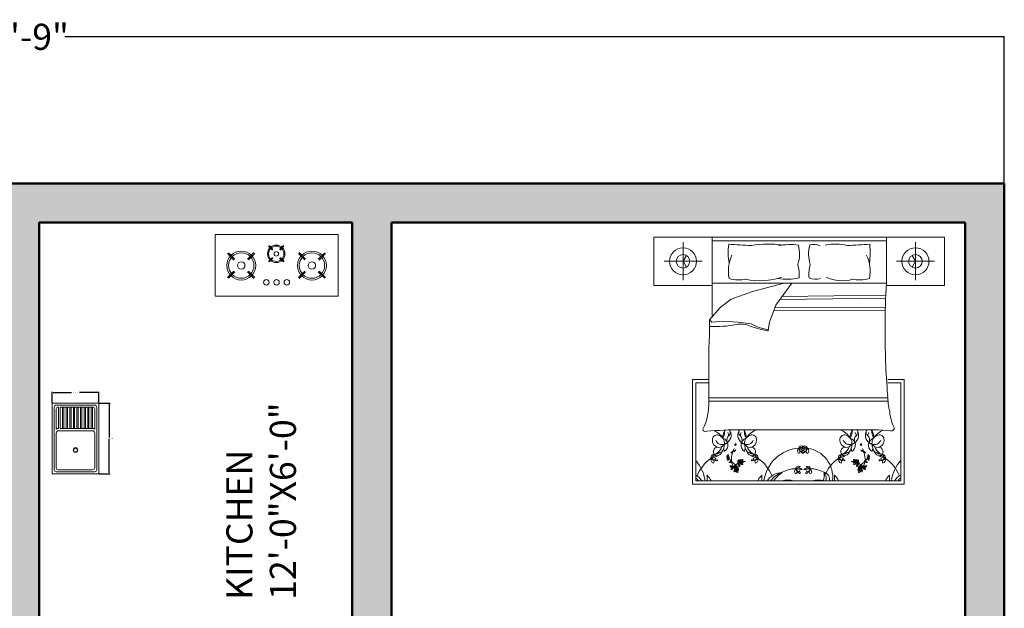
# Model space of a CAD drawing. Units: inches. Extents: x -17 to 536, y -817 to 53.
# Tile 9 of 9: x 268 to 494, y -86 to 49. Entities that reach past the tile are written whole.
import ezdxf

# ---------------------------------------------------------------- set-up
doc = ezdxf.new("R2010")
doc.units = ezdxf.units.IN
doc.header["$MEASUREMENT"] = 0
for name, color, linetype, lineweight in [('A-ANNO-DIMS', 2, 'Continuous', 18), ('A-AREA-IDEN', 7, 'Continuous', 18), ('A-EQPM', 8, 'Continuous', 18), ('A-FLOR-FIXT', 9, 'Continuous', 18), ('A-FURN', 8, 'Continuous', 13), ('A-WALL', 7, 'Continuous', 50), ('A-WALL-PATT', 22, 'Continuous', 13)]:
    doc.layers.add(name, color=color, linetype=linetype, lineweight=lineweight)
doc.styles.get("Standard").update_dxf_attribs({"font": 'arial.ttf'})
doc.dimstyles.get("Standard").update_dxf_attribs({"dimtxt": 0.18, "dimasz": 0.18, "dimexe": 0.18, "dimexo": 0.0625, "dimgap": 0.09, "dimtad": 0, "dimtih": 1, "dimtoh": 1, "dimdec": 0, "dimzin": 0, "dimdsep": 46, "dimlunit": 3, "dimtxsty": 'Standard', "dimcen": 0.09, "dimadec": 0, "dimazin": 0, "dimtfac": 1, "dimtdec": 0, "dimtofl": 0, "dimtmove": 0, "dimatfit": 3, "dimfxl": 1, "dimtolj": 1, "dimtzin": 0, "dimarcsym": 0})

# ---------------------------------------------------------------- blocks, each defined once
blk = doc.blocks.new('*D1')
at = {"layer": 'A-ANNO-DIMS', "color": 0, "lineweight": -2, "transparency": 16777216}
for p, q in [((41.37, 11.61), (41.37, 45.45)), ((494.37, 11.61), (494.37, 45.45)), ((41.55, 45.27), (257.47, 45.27)), ((494.19, 45.27), (278.26, 45.27))]:
    blk.add_line(p, q, dxfattribs=at)
at = {"layer": 'A-ANNO-DIMS', "color": 0, "transparency": 16777216}
for points in [[(41.55, 45.3), (41.55, 45.24), (41.37, 45.27)], [(494.19, 45.3), (494.19, 45.24), (494.37, 45.27)]]:
    blk.add_solid(points, dxfattribs=at)
at = {"layer": 'Defpoints', "color": 0, "transparency": 16777216}
for p in [(494.37, 45.27), (41.37, 11.55), (494.37, 11.55)]:
    blk.add_point(p, dxfattribs=at)
at = {"layer": 'A-ANNO-DIMS', "color": 0, "transparency": 16777216, "insert": (267.87, 45.27), "char_height": 6, "attachment_point": 5}
blk.add_mtext('\\A1;37\'-9"', dxfattribs=at)
blk = doc.blocks.new('М12 540х820')
for p, q in [((0, 540), (-820, 540)), ((-820, 540), (-820, 0)), ((-798, 495), (-798, 45)), ((-45, 517), (-775, 517)), ((-775, 468), (-775, 72)), ((-348, 495), (-748, 495)), ((-320, 468), (-320, 72)), ((-302, 495), (-65, 495)), ((-294, 468), (-294, 472)), ((-294, 468), (-45, 468)), ((-45, 470), (-45, 468)), ((-22, 45), (-22, 495)), ((0, 0), (0, 540)), ((-294, 447), (-45, 447)), ((-294, 420), (-294, 447)), ((-294, 420), (-45, 420)), ((-294, 405), (-45, 405)), ((-294, 378), (-294, 405)), ((-294, 378), (-45, 378)), ((-294, 336), (-294, 363)), ((-294, 363), (-45, 363)), ((-45, 420), (-45, 447)), ((-45, 378), (-45, 405)), ((-45, 336), (-45, 363)), ((-294, 336), (-45, 336)), ((-294, 295), (-294, 322)), ((-294, 322), (-45, 322)), ((-294, 295), (-45, 295)), ((-294, 253), (-294, 280)), ((-294, 280), (-45, 280)), ((-294, 253), (-45, 253)), ((-294, 211), (-294, 238)), ((-294, 238), (-45, 238)), ((-45, 295), (-45, 322)), ((-45, 253), (-45, 280)), ((-45, 211), (-45, 238)), ((-294, 211), (-45, 211)), ((-294, 170), (-294, 197)), ((-294, 197), (-45, 197)), ((-294, 170), (-45, 170)), ((-294, 128), (-294, 155)), ((-294, 155), (-45, 155)), ((-294, 128), (-45, 128)), ((-45, 170), (-45, 197)), ((-45, 128), (-45, 155)), ((-820, 0), (0, 0)), ((-775, 22), (-45, 22)), ((-748, 45), (-348, 45)), ((-302, 45), (-65, 45)), ((-294, 114), (-45, 114)), ((-294, 87), (-294, 114)), ((-294, 87), (-45, 87)), ((-294, 72), (-45, 72)), ((-45, 87), (-45, 114)), ((-45, 70), (-45, 72))]:
    blk.add_line(p, q)
at = {"ltscale": 0.06}
for p, q in [((-820, 0), (-820, 540)), ((-820, 540), (0, 540)), ((0, 540), (0, 537)), ((0, 537), (0, 0)), ((-294, 447), (-45, 447)), ((-294, 405), (-294, 447)), ((-294, 363), (-294, 405)), ((-294, 322), (-294, 363)), ((-45, 447), (-45, 420)), ((-45, 420), (-45, 378)), ((-45, 378), (-45, 336)), ((-294, 280), (-294, 322)), ((-294, 238), (-294, 280)), ((-294, 197), (-294, 238)), ((-45, 336), (-45, 295)), ((-45, 295), (-45, 253)), ((-45, 253), (-45, 211)), ((-294, 155), (-294, 197)), ((-294, 114), (-294, 155)), ((-45, 211), (-45, 170)), ((-45, 170), (-45, 128)), ((-45, 128), (-45, 87)), ((0, 0), (-820, 0)), ((-294, 72), (-294, 114)), ((-45, 72), (-294, 72)), ((-45, 87), (-45, 72))]:
    blk.add_line(p, q, dxfattribs=at)
at = {"extrusion": (0, 0, -1)}
for centre, major_axis, start_param, end_param in [((-775, 495), (-15.9, 15.9), -0.785398, 0.785398), ((-775, 495), (-15.9, 15.9), -0.785398, 0.785398), ((-748, 468), (-19.1, -19.1), 0.785398, 2.356194), ((-748, 468), (-19.1, -19.1), 0.785398, 2.356194), ((-348, 468), (-19.1, 19.1), 0.785398, 2.356194), ((-348, 468), (-19.1, 19.1), 0.785398, 2.356194), ((-343, 468), (-35, 35), 1.779263, 2.356194), ((-343, 468), (-35, 35), 1.779263, 2.356192), ((-343, 468), (-35, 35), 2.356192, 2.356194), ((-72, 469), (-19.3, 19.3), 1.0328, 2.38382), ((-72, 469), (-19.3, 19.3), 1.0328, 1.064673), ((-72, 469), (-19.3, 19.3), 1.064673, 2.328569), ((-45, 495), (-15.9, -15.9), 2.356194, 3.926991), ((-45, 495), (-15.9, -15.9), 2.356194, 3.926991), ((-72, 469), (-19.3, 19.3), 2.328569, 2.38382), ((-545, 270), (-19.1, -19.1), 3.926991, 10.210176), ((-545, 270), (-19.1, -19.1), 3.926991, 10.210176), ((-545, 270), (-15.9, -15.9), 3.926991, 10.210176), ((-545, 270), (-15.9, -15.9), 3.926991, 10.210176), ((-775, 45), (-15.9, -15.9), 5.497787, 7.068583), ((-775, 45), (-15.9, -15.9), 5.497787, 7.068583), ((-748, 72), (-19.1, 19.1), 3.926991, 5.497787), ((-748, 72), (-19.1, 19.1), 3.926991, 5.497787), ((-348, 72), (-19.1, -19.1), 3.926991, 5.497787), ((-348, 72), (-19.1, -19.1), 3.926991, 5.497787), ((-343, 72), (-35, -35), 3.926991, 4.503922), ((-343, 72), (-35, -35), 3.926991, 4.503922), ((-72, 71), (-19.3, -19.3), 3.899365, 5.250385), ((-72, 71), (-19.3, -19.3), 5.218512, 5.250385), ((-72, 71), (-19.3, -19.3), 3.954617, 5.218512), ((-72, 71), (-19.3, -19.3), 3.899365, 3.954617), ((-45, 45), (-15.9, 15.9), 2.356194, 3.926991), ((-45, 45), (-15.9, 15.9), 2.356194, 3.926991)]:
    blk.add_ellipse(centre, major_axis=major_axis, ratio=1, start_param=start_param, end_param=end_param, dxfattribs=at)
blk = doc.blocks.new('BED-WITH-NIGHTSTANDS-COMPACT')
for p, q in [((0, 56.83), (66.83, 56.83)), ((13.37, 56.83), (13.37, 38.49)), ((6.68, 46.9), (6.68, 55.63)), ((53.46, 55.97), (13.37, 55.97)), ((60.14, 46.9), (60.14, 55.63)), ((11.05, 51.26), (2.32, 51.26)), ((55.78, 51.26), (64.51, 51.26)), ((13.37, 46.27), (53.46, 46.27)), ((22.65, 44.28), (29.94, 46.27)), ((31.72, 46.27), (28.06, 41.17)), ((17.78, 42.53), (22.65, 44.28)), ((53.28, 43.49), (29.49, 43.16)), ((15.2, 40.63), (17.78, 42.53)), ((28.06, 41.17), (26.57, 37.25)), ((53.26, 42.81), (28.99, 42.47)), ((12.77, 37.79), (15.2, 40.63)), ((53.23, 40.02), (27.58, 39.91)), ((53.22, 40.7), (27.85, 40.6)), ((13.31, 37.25), (12.77, 37.79)), ((16.02, 37.52), (13.31, 37.25)), ((19.4, 37.25), (16.02, 37.52)), ((22.38, 36.85), (19.4, 37.25)), ((24.14, 36.03), (22.38, 36.85)), ((26.57, 37.25), (26.3, 35.49)), ((26.3, 35.49), (24.14, 36.03)), ((8.82, 24.07), (12.6, 24.07)), ((8.82, 0), (8.82, 24.07)), ((12.6, 23.3), (9.59, 23.3)), ((9.59, 23.3), (9.59, 0.77)), ((56.77, 23.3), (53.82, 23.3)), ((53.83, 24.07), (57.54, 24.07)), ((56.77, 0.77), (56.77, 23.3)), ((57.54, 24.07), (57.54, 0)), ((53.77, 19.9), (12.6, 19.9)), ((53.83, 19.07), (12.6, 19.07)), ((46.98, 12.51), (19.85, 12.51)), ((16.18, 7.55), (16.03, 8.3)), ((20.85, 7.55), (21, 8.3)), ((45.51, 7.55), (45.36, 8.3)), ((50.18, 7.55), (50.33, 8.3)), ((9.59, 0.77), (56.77, 0.77)), ((57.54, 0), (8.82, 0))]:
    blk.add_line(p, q)
for points in [[(13.37, 45.69), (0, 45.69), (0, 56.83)], [(53.46, 56.83), (53.46, 45.69), (66.83, 45.69), (66.83, 56.83)], [(6.68, 51.26), (7.46, 52.61)], [(60.14, 51.26), (59.36, 52.61)], [(6.68, 51.26), (7.46, 49.91)], [(60.14, 51.26), (59.36, 49.91)]]:
    blk.add_lwpolyline(points)
for points in [[(17.2, 55.17, 0.074897), (17.28, 50.8, -0.472817)], [(33.1, 50.56, 0.14099), (33.23, 55.01, 0.235245)], [(35.95, 50.56, -0.14099), (35.82, 55.01, -0.235245)], [(49.62, 55.17, -0.074897), (49.54, 50.8, 0.472817)], [(12.63, 31.67, 0.001242), (12.6, 18.99, -0.127202), (11.26, 12.67)], [(53.75, 20.43, 0.056112), (54.23, 16.75, 0.095341), (55.17, 13.21)]]:
    blk.add_lwpolyline(points, format="xyb")
for centre, radius in [((6.68, 51.26), 3.12), ((60.14, 51.26), 3.12), ((6.68, 51.26), 1.56), ((60.14, 51.26), 1.56), ((20.04, 5.13), 0.17), ((46.32, 5.13), 0.17), ((18.93, 3.33), 0.17), ((47.43, 3.33), 0.17)]:
    blk.add_circle(centre, radius)
for centre, radius, start, end in [((54.04, 691.14), 637.04, 266.68521, 267.14978), ((26.36, 30.98), 24.24, 82.2196, 99.497), ((31.48, 43.23), 11.91, 81.5249, 103.96), ((36.74, 51.83), 3.31, 63.3437, 106.1026), ((41.69, 43.47), 11.75, 76.3427, 101.1841), ((12.79, 691.14), 637.04, 272.85022, 273.31479), ((25.72, 49.05), 8.61, 155.1316, 191.7583), ((41.11, 49.05), 8.61, 348.2417, 24.8684), ((25.22, 48.32), 8.19, 354.0129, 15.8293), ((43.83, 48.32), 8.19, 164.1707, 185.9871), ((24.3, 62.31), 15.53, 258.0397, 289.2615), ((43.37, 55.29), 8.51, 243.8761, 286.1746), ((19.59, 55.95), 8.96, 255.1039, 281.0369), ((30.59, 58.92), 11.78, 259.8617, 283.6238), ((37.18, 50.68), 3.54, 245.0183, 288.5407), ((47.24, 55.95), 8.96, 258.9631, 284.8961), ((173.26, 38.1), 120.08, 176.1, 180.9282), ((-48.51, 36.13), 61.3, 355.8294, 1.553), ((13.91, 61.46), 25.22, 267.4519, 281.3392), ((19.94, 31.39), 5.44, 66.2616, 101.3392), ((30.94, 60.75), 25.92, 250.1194, 259.3383), ((26.15, 35.44), 0.161, 268.8623, 19.7536), ((209.82, 33.74), 156.63, 179.1145, 184.8735), ((11.87, 12.72), 0.617, 183.98, 297.3412), ((19.05, -57.06), 69.57, 89.3433, 95.6887), ((14.56, 10.23), 1.13, 84.4856, 181.0538), ((11.61, 7.8), 5.06, 33.6671, 63.2997), ((14.21, 9.39), 2.01, 355.2933, 76.921), ((18.39, 10.81), 2.58, 145.785, 184.7304), ((13.47, 12.01), 2.77, 328.8218, 9.1554), ((16.89, 11.77), 0.805, 120.0293, 142.325), ((15.61, 11.29), 2.13, 289.2822, 29.1751), ((15.29, 10.91), 1.92, 7.436, 29.9149), ((16.55, 11.93), 1, 311.5653, 23.8354), ((16.89, 11.77), 0.805, 44.4517, 63.558), ((21.42, 11.29), 2.13, 150.8249, 250.7178), ((20.48, 11.93), 1, 156.1646, 228.4347), ((20.14, 11.77), 0.805, 113.229, 135.5483), ((21.74, 10.91), 1.92, 150.0851, 172.564), ((20.14, 11.77), 0.805, 37.675, 66.7144), ((18.64, 10.81), 2.58, 355.2696, 34.215), ((23.57, 12.01), 2.77, 169.7133, 211.1782), ((22.82, 9.39), 2.01, 103.079, 184.7067), ((25.42, 7.8), 5.06, 111.4941, 146.3329), ((22.47, 10.23), 1.13, 358.9462, 95.5144), ((43.89, 10.23), 1.13, 84.4856, 181.0538), ((40.94, 7.8), 5.06, 33.6671, 68.5059), ((43.54, 9.39), 2.01, 355.2933, 76.921), ((47.72, 10.81), 2.58, 145.785, 184.7304), ((42.79, 12.01), 2.77, 328.8218, 10.2867), ((46.22, 11.77), 0.805, 113.2856, 142.325), ((44.94, 11.29), 2.13, 289.2822, 29.1751), ((44.62, 10.91), 1.92, 7.436, 29.9149), ((46.22, 11.77), 0.805, 44.4517, 66.7144), ((45.88, 11.93), 1, 311.5653, 23.8354), ((49.03, -52.49), 65.03, 85.2402, 91.8035), ((50.75, 11.29), 2.13, 150.8249, 250.7178), ((49.81, 11.93), 1, 156.1646, 228.4347), ((49.47, 11.77), 0.805, 106.6343, 135.5483), ((51.07, 10.91), 1.92, 150.0851, 172.564), ((49.47, 11.77), 0.805, 37.675, 72.5814), ((47.97, 10.81), 2.58, 355.2696, 34.215), ((52.9, 12.01), 2.77, 169.249, 211.1782), ((52.15, 9.39), 2.01, 103.079, 184.7067), ((54.75, 7.8), 5.06, 113.6453, 146.3329), ((51.8, 10.23), 1.13, 358.9462, 95.5144), ((54.66, 12.87), 0.609, 246.5219, 33.8264), ((15.02, 10.07), 1.6, 174.9449, 262.8857), ((15.65, 10.67), 1.55, 201.5819, 291.4221), ((14.74, 10.42), 1.94, 272.3591, 324.0401), ((12.63, 9.45), 3.59, 326.2883, 356.5076), ((15.35, 8.99), 1.66, 299.9085, 73.1337), ((18.39, 10.81), 2.58, 212.7011, 216.3445), ((16.4, 9.69), 0.415, 257.3041, 15.1471), ((18.13, 10.15), 1.37, 131.5653, 195.1471), ((18.71, 9.06), 0.129, 102.7051, 280.4384), ((18.69, 9.14), 0.209, 280.4384, 100.4136), ((18.9, 10.15), 1.37, 344.8529, 48.4347), ((21.68, 8.99), 1.66, 106.8663, 240.0915), ((20.63, 9.69), 0.415, 164.8529, 282.6959), ((18.64, 10.81), 2.58, 323.6555, 327.2989), ((22.29, 10.42), 1.94, 215.9599, 267.6409), ((21.38, 10.67), 1.55, 248.5779, 338.4181), ((24.4, 9.45), 3.59, 183.4924, 213.7117), ((22.01, 10.07), 1.6, 277.1143, 5.0551), ((44.35, 10.07), 1.6, 174.9449, 262.8857), ((44.98, 10.67), 1.55, 201.5819, 291.4221), ((44.07, 10.42), 1.94, 272.3591, 324.0401), ((41.96, 9.45), 3.59, 326.2883, 356.5076), ((44.68, 8.99), 1.66, 299.9085, 73.1337), ((47.72, 10.81), 2.58, 212.7011, 216.3445), ((45.73, 9.69), 0.415, 257.3041, 15.1471), ((47.46, 10.15), 1.37, 131.5653, 195.1471), ((47.67, 9.14), 0.209, 79.5864, 259.5616), ((47.65, 9.06), 0.129, 259.5616, 77.2949), ((48.23, 10.15), 1.37, 344.8529, 48.4347), ((51.01, 8.99), 1.66, 106.8663, 240.0915), ((49.96, 9.69), 0.415, 164.8529, 282.6959), ((47.97, 10.81), 2.58, 323.6555, 327.2989), ((51.62, 10.42), 1.94, 215.9599, 267.6409), ((50.71, 10.67), 1.55, 248.5779, 338.4181), ((53.73, 9.45), 3.59, 183.4924, 213.7117), ((51.34, 10.07), 1.6, 277.1143, 5.0551), ((13.8, 6.11), 0.723, 92.9516, 193.728), ((12.32, 7.21), 1.49, 301.3827, 345.2969), ((14.65, 7.5), 1, 80.264, 250.8688), ((14.45, 6.41), 0.615, 63.9755, 143.2681), ((12.66, 9.7), 3.15, 301.2614, 341.7045), ((14.41, 7.8), 1.25, 265.969, 344.3045), ((15.76, 6.13), 1.33, 96.1662, 141.5825), ((17.97, 7.07), 0.351, 101.3256, 154.4621), ((17.46, 8.26), 1.06, 280.2588, 300.656), ((17.71, 9.1), 1.88, 268.3264, 277.1302), ((23.34, 5.69), 5.53, 163.5842, 183.8277), ((17.24, 8.26), 1.07, 308.2101, 316.3071), ((17.9, 7.55), 0.321, 278.3432, 4.2869), ((17.72, 7.83), 0.56, 300.656, 332.6341), ((18.14, 7.46), 0.136, 55.7657, 157.4417), ((23.34, 5.69), 5.53, 153.0032, 159.8941), ((18.35, 7.59), 0.136, 84.3784, 186.0543), ((18.22, 8.13), 0.56, 269.1859, 301.164), ((18.39, 7.84), 0.321, 237.5332, 323.4768), ((18.08, 8.76), 1.07, 285.5129, 293.6099), ((17.97, 8.56), 1.06, 301.164, 321.5612), ((18.78, 7.55), 0.351, 87.3579, 140.4944), ((17.11, 8.74), 1.88, 324.6898, 333.4936), ((24.37, 9.7), 3.15, 198.2955, 238.7386), ((21.27, 6.13), 1.33, 38.4175, 83.8338), ((22.62, 7.8), 1.25, 195.6955, 274.031), ((22.38, 7.5), 1, 289.1312, 99.736), ((22.59, 6.41), 0.615, 36.7319, 116.0245), ((23.23, 6.11), 0.723, 346.272, 87.0484), ((24.71, 7.21), 1.49, 194.7031, 238.6173), ((33.93, -0.4), 8.73, 94.4623, 172.255), ((33.97, 7.65), 0.968, 137.7873, 219.1145), ((32.87, 7.68), 0.729, 298.5391, 58.3627), ((33.95, 8.1), 0.723, 63.0274, 163.8037), ((33.22, 9.79), 1.49, 271.4585, 315.3727), ((33.82, 7.04), 1.38, 45.5411, 114.3101), ((35.08, 14.12), 6.1, 252.593, 267.2582), ((33.97, 8.27), 0.714, 177.7585, 283.852), ((35.34, 9.01), 2.21, 198.9159, 238.011), ((34.77, 7.04), 1.38, 65.6899, 134.4589), ((33.51, 14.12), 6.1, 272.7418, 287.407), ((34.12, 7.67), 0.0944, 283.852, 219.9245), ((34.23, 7.23), 0.108, 238.011, 71.5592), ((34.25, 7.29), 0.0526, 71.5592, 188.0167), ((34.36, 7.23), 0.108, 108.4408, 301.989), ((34.64, 8.1), 0.723, 16.1963, 116.9726), ((35.37, 9.79), 1.49, 224.6273, 268.5415), ((34.34, 7.29), 0.0526, 351.9833, 108.4408), ((34.46, 7.71), 0.0569, 320.1909, 256.0209), ((33.25, 9.01), 2.21, 301.989, 341.0841), ((34.62, 8.27), 0.714, 256.148, 2.2415), ((35.72, 7.68), 0.729, 121.6373, 241.4609), ((34.62, 7.65), 0.968, 320.8855, 42.2127), ((34.37, 1.61), 6.75, 352.8636, 81.8197), ((43.13, 6.11), 0.723, 92.9516, 193.728), ((41.65, 7.21), 1.49, 301.3827, 345.2969), ((43.98, 7.5), 1, 80.264, 250.8688), ((43.77, 6.41), 0.615, 63.9755, 143.2681), ((41.99, 9.7), 3.15, 301.2614, 341.7045), ((43.74, 7.8), 1.25, 265.969, 344.3045), ((45.09, 6.13), 1.33, 96.1662, 141.5825), ((48.39, 8.56), 1.06, 218.4388, 238.836), ((47.58, 7.55), 0.351, 39.5056, 92.6421), ((49.25, 8.74), 1.88, 206.5064, 215.3102), ((47.97, 7.84), 0.321, 216.5232, 302.4668), ((48.28, 8.76), 1.07, 246.3901, 254.4871), ((48.14, 8.13), 0.56, 238.836, 270.8141), ((43.02, 5.69), 5.53, 20.1059, 26.9968), ((48.01, 7.59), 0.136, 353.9457, 95.6216), ((48.47, 7.55), 0.321, 175.7131, 261.6568), ((48.22, 7.46), 0.136, 22.5583, 124.2343), ((48.64, 7.83), 0.56, 207.3659, 239.344), ((43.02, 5.69), 5.53, 356.1723, 16.4158), ((49.12, 8.26), 1.07, 223.6929, 231.7899), ((48.9, 8.26), 1.06, 239.344, 259.7412), ((48.65, 9.1), 1.88, 262.8698, 271.6736), ((48.39, 7.07), 0.351, 25.5379, 78.6744), ((53.7, 9.7), 3.15, 198.2955, 238.7386), ((51.95, 7.8), 1.25, 195.6955, 274.031), ((50.6, 6.13), 1.33, 38.4175, 83.8338), ((51.71, 7.5), 1, 289.1312, 99.736), ((51.92, 6.41), 0.615, 36.7319, 116.0245), ((54.04, 7.21), 1.49, 194.7031, 238.6173), ((52.56, 6.11), 0.723, 346.272, 87.0484), ((3.1, -0.4), 8.73, 7.745, 41.8856), ((18.03, -1.26), 8.73, 124.3865, 158.5908), ((14.05, 5.73), 0.968, 167.7115, 249.0387), ((14.22, 5.13), 1.38, 75.4653, 144.2343), ((11.78, 11.9), 6.1, 282.5173, 297.1824), ((13.08, 5.21), 0.729, 328.4633, 88.2869), ((14.55, 7.6), 2.21, 228.8402, 267.9352), ((13.73, 6.27), 0.714, 207.6827, 313.7762), ((14.16, 5.82), 0.0944, 313.7762, 249.7183), ((14.47, 5.56), 0.0526, 101.4834, 217.9409), ((14.48, 5.5), 0.108, 267.9352, 101.4834), ((16.98, 6.4), 0.284, 101.5637, 142.6358), ((16.74, 6.14), 0.17, 273.2768, 86.7232), ((16.97, 5.82), 0.281, 217.7621, 259.0403), ((16.94, 6.3), 0.163, 91.1081, 181.8675), ((17.28, 6.2), 0.517, 203.4276, 227.6104), ((17.11, 5.97), 0.352, 80.3487, 133.6538), ((17.05, 6.26), 0.278, 229.7889, 317.6792), ((16.75, 6.63), 0.409, 288.7263, 352.5032), ((16.74, 5.67), 0.395, 355.053, 68.3618), ((17.05, 5.61), 0.557, 83.0852, 105.7171), ((17.03, 6.61), 0.131, 345.2356, 144.9248), ((17, 5.65), 0.131, 232.4737, 355.053), ((13.19, 0.99), 6.35, 43.1541, 52.0459), ((17.15, 6.18), 0.147, 317.6792, 80.3487), ((17.57, 4.82), 0.351, 101.3256, 154.4621), ((17.07, 6.01), 1.06, 280.2588, 300.656), ((17.31, 6.85), 1.88, 268.3264, 277.1302), ((16.84, 6.01), 1.07, 308.2101, 316.3071), ((17.5, 5.3), 0.321, 278.3432, 4.2869), ((17.74, 5.21), 0.136, 55.7657, 157.4417), ((17.32, 5.58), 0.56, 300.656, 332.6341), ((20.58, 5.56), 2.77, 184.756, 209.2041), ((24.58, 11.46), 9.13, 222.2412, 232.1744), ((20.87, 1.87), 3.33, 120.544, 139.818), ((18.74, 5.38), 0.776, 304.5369, 16.3699), ((19.15, 5.21), 0.472, 272.8499, 356.1226), ((18.82, 5.02), 0.457, 321.7607, 7.9252), ((18.92, 4.37), 0.457, 8.7227, 54.8872), ((18.94, 4), 0.776, 0.278, 72.111), ((19.82, 5.16), 0.549, 127.3105, 187.9252), ((19.29, 4.29), 0.472, 20.5253, 88.5375), ((19.06, 5.22), 0.564, 355.0106, 41.658), ((19.68, 4.81), 0.169, 148.0499, 225.6268), ((20.87, 1.87), 3.33, 113.0501, 113.8477), ((20, 4.61), 0.537, 104.7558, 148.0499), ((19.69, 5), 0.336, 247.4086, 351.4386), ((19.85, 5.36), 0.232, 126.1046, 271.4281), ((19.83, 5.43), 0.167, 353.7526, 131.7054), ((19.67, 5.23), 0.234, 0.0645, 61.1507), ((19.79, 4.98), 0.113, 262.906, 7.132), ((19.73, 5.43), 0.268, 311.8413, 355.7877), ((20.28, 5.39), 0.284, 101.5637, 176.365), ((20.27, 4.81), 0.281, 151.2196, 259.0403), ((20.24, 5.29), 0.163, 91.1081, 181.8675), ((20.58, 5.19), 0.517, 203.4276, 227.6104), ((20.41, 4.96), 0.352, 80.3487, 133.6538), ((20.35, 5.25), 0.278, 229.7889, 317.6792), ((20.05, 5.61), 0.409, 288.7263, 352.5032), ((20.04, 4.66), 0.395, 355.053, 68.3618), ((20.35, 4.6), 0.557, 83.0852, 105.7171), ((20.33, 5.59), 0.131, 345.2356, 144.9248), ((20.3, 4.64), 0.131, 232.4737, 355.053), ((20.45, 5.16), 0.147, 317.6792, 80.3487), ((20.87, 1.87), 3.33, 87.1071, 94.7585), ((22.55, 5.5), 0.108, 78.5166, 272.0648), ((22.81, 5.13), 1.38, 35.7657, 104.5347), ((25.25, 11.9), 6.1, 242.8176, 257.4827), ((22.48, 7.6), 2.21, 272.0648, 311.1598), ((22.57, 5.56), 0.0526, 322.0591, 78.5166), ((23.3, 6.27), 0.714, 226.2238, 332.3173), ((22.88, 5.86), 0.0569, 290.2667, 226.2271), ((23.95, 5.21), 0.729, 91.7131, 211.5367), ((22.99, 5.73), 0.968, 290.9613, 12.2885), ((19, -1.26), 8.73, 21.4092, 55.6135), ((47.36, -1.26), 8.73, 124.3865, 158.5908), ((43.37, 5.73), 0.968, 167.7115, 249.0387), ((43.55, 5.13), 1.38, 75.4653, 144.2343), ((41.11, 11.9), 6.1, 282.5173, 297.1824), ((43.06, 6.27), 0.714, 207.6827, 313.7762), ((43.88, 7.6), 2.21, 228.8402, 267.9352), ((42.41, 5.21), 0.729, 328.4633, 88.2869), ((43.49, 5.82), 0.0944, 313.7762, 249.7183), ((43.79, 5.56), 0.0526, 101.4834, 217.9409), ((43.81, 5.5), 0.108, 267.9352, 101.4834), ((45.49, 1.87), 3.33, 85.2415, 92.8929), ((45.91, 5.16), 0.147, 99.6513, 222.3208), ((46.01, 5.25), 0.278, 222.3208, 310.2111), ((45.95, 4.96), 0.352, 46.3462, 99.6513), ((46.03, 5.59), 0.131, 35.0752, 194.7644), ((46.31, 5.61), 0.409, 187.4968, 251.2737), ((46.33, 4.66), 0.395, 111.6382, 184.947), ((46.06, 4.64), 0.131, 184.947, 307.5263), ((46.02, 4.6), 0.557, 74.2829, 96.9148), ((46.12, 5.29), 0.163, 358.1325, 88.8919), ((45.78, 5.19), 0.517, 312.3896, 336.5724), ((46.08, 5.39), 0.284, 3.635, 78.4363), ((46.09, 4.81), 0.281, 280.9597, 28.7804), ((46.67, 5), 0.336, 188.5614, 292.5914), ((46.53, 5.43), 0.167, 48.2946, 186.2474), ((46.63, 5.43), 0.268, 184.2123, 228.1587), ((46.69, 5.23), 0.234, 118.8493, 179.9355), ((46.57, 4.98), 0.113, 172.868, 277.094), ((46.51, 5.36), 0.232, 268.5719, 53.8954), ((46.36, 4.61), 0.537, 31.9501, 75.2442), ((47.07, 4.29), 0.472, 91.4625, 159.4747), ((47.42, 4), 0.776, 107.889, 179.722), ((47.3, 5.22), 0.564, 138.342, 184.9894), ((47.21, 5.21), 0.472, 183.8774, 267.1501), ((45.49, 1.87), 3.33, 66.1523, 66.9499), ((46.68, 4.81), 0.169, 314.3732, 31.9501), ((47.62, 5.38), 0.776, 163.6301, 235.4631), ((46.55, 5.16), 0.549, 352.0748, 52.6895), ((47.45, 4.37), 0.457, 125.1128, 171.2773), ((47.54, 5.02), 0.457, 172.0748, 218.2393), ((45.49, 1.87), 3.33, 40.182, 59.456), ((41.78, 11.46), 9.13, 307.8256, 317.7588), ((45.78, 5.56), 2.77, 330.7959, 355.244), ((53.17, 0.99), 6.35, 127.9541, 136.8459), ((48.62, 5.21), 0.136, 22.5583, 124.2343), ((48.86, 5.3), 0.321, 175.7131, 261.6568), ((49.04, 5.58), 0.56, 207.3659, 239.344), ((49.52, 6.01), 1.07, 223.6929, 231.7899), ((49.29, 6.01), 1.06, 239.344, 259.7412), ((49.05, 6.85), 1.88, 262.8698, 271.6736), ((48.79, 4.82), 0.351, 25.5379, 78.6744), ((49.21, 6.18), 0.147, 99.6513, 222.3208), ((49.31, 6.26), 0.278, 222.3208, 310.2111), ((49.25, 5.97), 0.352, 46.3462, 99.6513), ((49.33, 6.61), 0.131, 35.0752, 194.7644), ((49.61, 6.63), 0.409, 187.4968, 251.2737), ((49.62, 5.67), 0.395, 111.6382, 184.947), ((49.36, 5.65), 0.131, 184.947, 307.5263), ((49.31, 5.61), 0.557, 74.2829, 96.9148), ((49.42, 6.3), 0.163, 358.1325, 88.8919), ((49.08, 6.2), 0.517, 312.3896, 336.5724), ((49.38, 6.4), 0.284, 37.3642, 78.4363), ((49.39, 5.82), 0.281, 280.9597, 322.2379), ((49.62, 6.14), 0.17, 93.2768, 266.7232), ((51.88, 5.5), 0.108, 78.5166, 272.0648), ((52.14, 5.13), 1.38, 35.7657, 104.5347), ((54.58, 11.9), 6.1, 242.8176, 257.4827), ((51.81, 7.6), 2.21, 272.0648, 311.1598), ((51.9, 5.56), 0.0526, 322.0591, 78.5166), ((52.63, 6.27), 0.714, 226.2238, 332.3173), ((52.21, 5.86), 0.0569, 290.2667, 226.2271), ((53.28, 5.21), 0.729, 91.7131, 211.5367), ((52.32, 5.73), 0.968, 290.9613, 12.2885), ((48.33, -1.26), 8.73, 21.4092, 55.6135), ((63.26, -0.4), 8.73, 138.1144, 172.255), ((17.69, 4.2), 0.19, 146.8636, 236.9021), ((20.37, 8.39), 4.97, 235.1882, 238.8844), ((18.02, 4.48), 0.514, 199.4799, 267.6828), ((17.96, 4.28), 0.443, 212.8155, 277.3992), ((17.7, 3.99), 0.514, 266.9701, 338.2913), ((14.99, 7.66), 4.97, 302.6784, 306.3746), ((17.83, 3.58), 0.19, 214.3538, 304.3923), ((17.9, 4.3), 0.197, 238.8844, 314.2646), ((17.86, 3.86), 0.443, 280.3057, 17.1958), ((17.82, 3.81), 0.197, 306.3746, 21.7548), ((18.14, 3.94), 0.148, 19.3605, 201.7548), ((18.14, 4.05), 0.148, 311.8703, 134.2646), ((20.93, 2.7), 2.96, 153.7819, 158.2913), ((18.57, 4.73), 0.776, 247.2305, 319.0635), ((18.32, 4.47), 0.457, 264.4544, 310.6188), ((20.58, 5.56), 2.77, 214.0033, 222.4917), ((18.65, 4.28), 0.472, 218.3208, 298.8162), ((18.57, 3.01), 0.169, 148.0499, 225.6268), ((18.88, 2.82), 0.537, 104.7558, 148.0499), ((18.58, 3.2), 0.336, 247.4086, 351.4386), ((18.74, 3.57), 0.232, 126.1046, 271.4281), ((18.71, 3.63), 0.167, 353.7526, 131.7054), ((18.97, 3.7), 0.549, 70.0041, 130.6188), ((18.68, 3.19), 0.113, 262.906, 7.132), ((18.56, 3.44), 0.234, 0.0645, 61.1507), ((18.61, 3.64), 0.268, 311.8413, 355.7877), ((18.62, 4.37), 0.564, 297.7043, 344.3516), ((19.16, 3.6), 0.284, 101.5637, 176.365), ((19.16, 3.02), 0.281, 151.2196, 259.0403), ((19.13, 3.49), 0.163, 91.1081, 181.8675), ((19.46, 3.39), 0.517, 203.4276, 227.6104), ((19.3, 3.17), 0.352, 80.3487, 133.6538), ((19.24, 3.46), 0.278, 229.7889, 317.6792), ((18.94, 3.82), 0.409, 288.7263, 352.5032), ((18.92, 2.87), 0.395, 355.053, 68.3618), ((19.23, 2.8), 0.557, 83.0852, 105.7171), ((19.21, 3.8), 0.131, 345.2356, 144.9248), ((19.19, 2.85), 0.131, 232.4737, 355.053), ((19.33, 3.37), 0.147, 317.6792, 80.3487), ((19.91, 4.52), 0.549, 188.7227, 249.3375), ((19.2, 4.25), 0.564, 334.9899, 21.6373), ((29.56, -1.57), 4.25, 91.272, 146.5383), ((31.09, -2.36), 5.3, 107.8504, 143.6964), ((33.87, -3.85), 7.88, 124.0123, 144.053), ((33.26, -5.08), 8.73, 94.4623, 117.4146), ((33.3, 2.97), 0.968, 137.7873, 219.1145), ((32.2, 3), 0.729, 298.5391, 58.3627), ((33.28, 3.42), 0.723, 63.0274, 163.8037), ((32.55, 5.11), 1.49, 271.4585, 315.3727), ((33.15, 2.37), 1.38, 45.5411, 114.3101), ((34.67, 4.34), 2.21, 198.9159, 238.011), ((34.41, 9.45), 6.1, 252.593, 267.2582), ((33.3, 3.6), 0.714, 177.7585, 283.852), ((33.45, 2.99), 0.0944, 283.852, 219.9245), ((33.56, 2.56), 0.108, 238.011, 71.5592), ((33.58, 2.61), 0.0526, 71.5592, 188.0167), ((35.43, 2.37), 1.38, 65.6899, 134.4589), ((34.18, 9.45), 6.1, 272.7418, 287.407), ((35.03, 2.56), 0.108, 108.4408, 301.989), ((35.31, 3.42), 0.723, 16.1963, 116.9726), ((36.04, 5.11), 1.49, 224.6273, 268.5415), ((35.01, 2.61), 0.0526, 351.9833, 108.4408), ((35.13, 3.03), 0.0569, 320.1909, 256.0209), ((33.91, 4.34), 2.21, 301.989, 341.0841), ((35.29, 3.6), 0.714, 256.148, 2.2415), ((36.38, 3), 0.729, 121.6373, 241.4609), ((35.29, 2.97), 0.968, 320.8855, 42.2127), ((35.32, -5.08), 8.73, 62.5854, 85.5377), ((35.25, 2.23), 3.91, 338.117, 6.6195), ((38.83, 1.14), 1.57, 346.3898, 79.0739), ((37.65, 1.36), 1.98, 342.8609, 41.9049), ((47.16, 4.25), 0.564, 158.3627, 205.0101), ((46.45, 4.52), 0.549, 290.6625, 351.2773), ((47.03, 3.37), 0.147, 99.6513, 222.3208), ((47.12, 3.46), 0.278, 222.3208, 310.2111), ((47.06, 3.17), 0.352, 46.3462, 99.6513), ((47.15, 3.8), 0.131, 35.0752, 194.7644), ((47.43, 3.82), 0.409, 187.4968, 251.2737), ((47.44, 2.87), 0.395, 111.6382, 184.947), ((47.17, 2.85), 0.131, 184.947, 307.5263), ((47.13, 2.8), 0.557, 74.2829, 96.9148), ((47.39, 3.7), 0.549, 49.3812, 109.9959), ((47.79, 4.73), 0.776, 220.9365, 292.7695), ((47.74, 4.37), 0.564, 195.6484, 242.2957), ((47.23, 3.49), 0.163, 358.1325, 88.8919), ((47.2, 3.6), 0.284, 3.635, 78.4363), ((46.9, 3.39), 0.517, 312.3896, 336.5724), ((47.2, 3.02), 0.281, 280.9597, 28.7804), ((47.78, 3.2), 0.336, 188.5614, 292.5914), ((47.71, 4.28), 0.472, 241.1838, 321.6792), ((47.65, 3.63), 0.167, 48.2946, 186.2474), ((47.75, 3.64), 0.268, 184.2123, 228.1587), ((47.8, 3.44), 0.234, 118.8493, 179.9355), ((47.68, 3.19), 0.113, 172.868, 277.094), ((47.62, 3.57), 0.232, 268.5719, 53.8954), ((47.48, 2.82), 0.537, 31.9501, 75.2442), ((48.04, 4.47), 0.457, 229.3812, 275.5456), ((45.78, 5.56), 2.77, 317.5083, 325.9967), ((47.79, 3.01), 0.169, 314.3732, 31.9501), ((48.5, 3.86), 0.443, 162.8042, 259.6943), ((48.22, 4.05), 0.148, 45.7354, 228.1297), ((48.22, 3.94), 0.148, 338.2452, 160.6395), ((45.43, 2.7), 2.96, 21.7087, 26.2181), ((48.66, 3.99), 0.514, 201.7087, 273.0299), ((48.46, 4.3), 0.197, 225.7354, 301.1156), ((48.54, 3.81), 0.197, 158.2452, 233.6254), ((48.4, 4.28), 0.443, 262.6008, 327.1845), ((48.35, 4.48), 0.514, 272.3172, 340.5201), ((51.37, 7.66), 4.97, 233.6254, 237.3216), ((48.53, 3.58), 0.19, 235.6077, 325.6462), ((45.99, 8.39), 4.97, 301.1156, 304.8118), ((48.67, 4.2), 0.19, 303.0979, 33.1364), ((7.48, -1.57), 4.25, 33.4617, 60.1116), ((5.95, -2.36), 5.3, 36.3036, 46.4814), ((9.86, -0.59), 3.55, 22.5547, 48.9546), ((0.14, 1.32), 12.07, 357.4081, 3.6519), ((27.17, -0.59), 3.55, 131.0454, 157.4453), ((36.89, 1.32), 12.07, 176.3481, 182.5919), ((30.82, -3.81), 4.8, 73.5431, 107.0202), ((32.73, -6.29), 7.1, 94.3787, 95.6357), ((36.46, -11.15), 12.68, 109.7217, 109.9028), ((37.76, -3.81), 4.8, 72.9798, 106.4569), ((35.86, -6.29), 7.1, 84.3643, 85.6213), ((32.13, -11.15), 12.68, 70.0972, 70.2783), ((29.47, 1.32), 12.07, 357.4081, 3.6519), ((39.19, -0.59), 3.55, 22.5547, 48.9546), ((56.5, -0.59), 3.55, 131.0454, 157.4453), ((66.22, 1.32), 12.07, 176.3481, 182.5919), ((58.88, -1.57), 4.25, 119.8884, 146.5383), ((60.41, -2.36), 5.3, 133.5186, 143.6964)]:
    blk.add_arc(centre, radius, start, end)
blk = doc.blocks.new('COOKTOP-3-BURNER')
for p, q in [((28.32, 14.16), (0, 14.16)), ((0, 14.16), (0, 0)), ((28.32, 0), (28.32, 14.16)), ((13.21, 10.58), (12.33, 11.47)), ((13.33, 10.7), (12.44, 11.58)), ((14.86, 10.7), (15.74, 11.58)), ((14.97, 10.58), (15.86, 11.47)), ((4.36, 8.28), (2.89, 9.76)), ((4.56, 8.48), (3.08, 9.95)), ((7.48, 8.49), (8.95, 9.98)), ((7.68, 8.3), (9.14, 9.78)), ((20.64, 8.3), (19.18, 9.78)), ((20.84, 8.49), (19.38, 9.98)), ((23.76, 8.48), (25.24, 9.95)), ((23.96, 8.28), (25.43, 9.76)), ((13.2, 8.83), (12.31, 7.95)), ((13.32, 8.71), (12.43, 7.83)), ((14.86, 8.71), (15.76, 7.83)), ((14.98, 8.83), (15.87, 7.95)), ((4.36, 5.74), (2.89, 4.27)), ((4.56, 5.54), (3.08, 4.07)), ((7.48, 5.53), (8.95, 4.05)), ((7.68, 5.73), (9.14, 4.24)), ((20.64, 5.73), (19.18, 4.24)), ((20.84, 5.53), (19.38, 4.05)), ((23.76, 5.54), (25.24, 4.07)), ((23.96, 5.74), (25.43, 4.27)), ((0, 0), (28.32, 0))]:
    blk.add_line(p, q)
for centre, radius in [((14.09, 9.7), 2), ((14.09, 9.7), 1.76), ((6.03, 7.01), 3.33), ((6.03, 7.01), 2.93), ((14.09, 9.7), 0.515), ((22.29, 7.01), 3.33), ((22.29, 7.01), 2.93), ((6.03, 7.01), 0.858), ((22.29, 7.01), 0.858), ((11.8, 3.15), 0.629), ((14.16, 3.15), 0.629), ((16.52, 3.15), 0.629)]:
    blk.add_circle(centre, radius)
blk = doc.blocks.new('*D28')
at = {"layer": 'A-ANNO-DIMS', "color": 0, "lineweight": -2, "transparency": 16777216}
for p, q in [((286.11, -38.98), (288.65, -38.98)), ((288.47, -39.16), (288.47, -46.9)), ((288.47, -55.01), (288.47, -47.27)), ((286.11, -55.19), (288.65, -55.19))]:
    blk.add_line(p, q, dxfattribs=at)
at = {"layer": 'A-ANNO-DIMS', "color": 0, "transparency": 16777216}
for points in [[(288.44, -39.16), (288.5, -39.16), (288.47, -38.98)], [(288.44, -55.01), (288.5, -55.01), (288.47, -55.19)]]:
    blk.add_solid(points, dxfattribs=at)
at = {"layer": 'Defpoints', "color": 0, "transparency": 16777216}
for p in [(286.04, -38.98), (288.47, -38.98), (286.04, -55.19)]:
    blk.add_point(p, dxfattribs=at)
at = {"layer": 'A-ANNO-DIMS', "color": 0, "transparency": 16777216, "insert": (288.47, -47.08), "char_height": 0.18, "attachment_point": 5}
blk.add_mtext('\\A1;SINK 1\'-4" TYP.', dxfattribs=at)
blk = doc.blocks.new('*D29')
at = {"layer": 'A-ANNO-DIMS', "color": 0, "lineweight": -2, "transparency": 16777216}
for p, q in [((275.37, -38.92), (275.37, -36.37)), ((275.55, -36.55), (279.79, -36.55)), ((285.86, -36.55), (281.63, -36.55)), ((286.04, -38.92), (286.04, -36.37))]:
    blk.add_line(p, q, dxfattribs=at)
at = {"layer": 'A-ANNO-DIMS', "color": 0, "transparency": 16777216}
for points in [[(275.55, -36.52), (275.55, -36.58), (275.37, -36.55)], [(285.86, -36.52), (285.86, -36.58), (286.04, -36.55)]]:
    blk.add_solid(points, dxfattribs=at)
at = {"layer": 'Defpoints', "color": 0, "transparency": 16777216}
for p in [(275.37, -36.55), (275.37, -38.98), (286.04, -38.98)]:
    blk.add_point(p, dxfattribs=at)
at = {"layer": 'A-ANNO-DIMS', "color": 0, "transparency": 16777216, "insert": (280.71, -36.55), "char_height": 0.18, "attachment_point": 5}
blk.add_mtext('\\A1;0\'-10 1/2" TYP.', dxfattribs=at)

msp = doc.modelspace()

# ---------------------------------------------------------------- hatches: boundary and pattern name
at = {"layer": 'A-WALL-PATT'}
h = msp.add_hatch(color=256, dxfattribs=at)
h.dxf.hatch_style = 1
h.paths.add_polyline_path([(217.37, -544.45), (208.37, -544.45), (208.37, -775.45), (217.37, -775.45)], flags=17)
h.paths.add_polyline_path([(327.37, -544.45), (318.37, -544.45), (318.37, -775.45), (327.37, -775.45)], flags=17)
h.paths.add_polyline_path([(494.37, 11.55), (41.37, 11.55), (41.37, -775.45), (50.37, -775.45), (50.37, -739.45), (184.37, -739.45), (184.37, -730.45), (50.37, -730.45), (50.37, -610.45), (172.37, -610.45), (172.37, -601.45), (155.37, -601.45), (155.37, -577.45), (146.37, -577.45), (146.37, -601.45), (50.37, -601.45), (50.37, -553.45), (172.37, -553.45), (172.37, -544.45), (50.37, -544.45), (50.37, -436.45), (191.37, -436.45), (191.37, -319.45), (182.37, -319.45), (182.37, -427.45), (50.37, -427.45), (50.37, -283.45), (98.37, -283.45), (98.37, -274.45), (50.37, -274.45), (50.37, -219.45), (122.37, -219.45), (122.37, -283.45), (191.37, -283.45), (191.37, -274.45), (131.37, -274.45), (131.37, -219.45), (131.37, -150.45), (146.37, -150.45), (146.37, -141.45), (122.37, -141.45), (122.37, -210.45), (50.37, -210.45), (50.37, -150.45), (98.37, -150.45), (98.37, -141.45), (50.37, -141.45), (50.37, 2.55), (182.37, 2.55), (182.37, -150.45), (191.37, -150.45), (191.37, 2.55), (263.37, 2.55), (263.37, -141.45), (227.37, -141.45), (227.37, -150.45), (263.37, -150.45), (263.37, -553.45), (272.37, -553.45), (272.37, -150.45), (308.37, -150.45), (308.37, -141.45), (272.37, -141.45), (272.37, 2.55), (344.37, 2.55), (344.37, -150.45), (353.37, -150.45), (353.37, 2.55), (485.37, 2.55), (485.37, -141.45), (437.37, -141.45), (437.37, -150.45), (485.37, -150.45), (485.37, -210.45), (413.37, -210.45), (413.37, -141.45), (389.37, -141.45), (389.37, -150.45), (404.37, -150.45), (404.37, -219.45), (404.37, -274.45), (353.37, -274.45), (344.37, -274.45), (344.37, -283.45), (353.37, -283.45), (413.37, -283.45), (413.37, -219.45), (485.37, -219.45), (485.37, -274.45), (437.37, -274.45), (437.37, -283.45), (485.37, -283.45), (485.37, -427.45), (353.37, -427.45), (353.37, -319.45), (344.37, -319.45), (344.37, -436.45), (485.37, -436.45), (485.37, -544.45), (363.37, -544.45), (363.37, -553.45), (485.37, -553.45), (485.37, -601.45), (389.37, -601.45), (389.37, -577.45), (380.37, -577.45), (380.37, -601.45), (363.37, -601.45), (363.37, -610.45), (485.37, -610.45), (485.37, -730.45), (351.37, -730.45), (351.37, -739.45), (485.37, -739.45), (485.37, -775.45), (494.37, -775.45)])

# ---------------------------------------------------------------- linework, layer by layer
at = {"layer": 'A-WALL'}
for p, q in [((41.37, 11.55), (494.37, 11.55)), ((494.37, 11.55), (494.37, -775.45)), ((272.37, 2.55), (272.37, -141.45)), ((272.37, 2.55), (344.37, 2.55)), ((344.37, 2.55), (344.37, -150.45)), ((353.37, 2.55), (353.37, -150.45)), ((353.37, 2.55), (485.37, 2.55)), ((485.37, 2.55), (485.37, -141.45))]:
    msp.add_line(p, q, dxfattribs=at)

# ---------------------------------------------------------------- block references
at = {"layer": 'A-EQPM'}
msp.add_blockref('COOKTOP-3-BURNER', (312.8, -14.33), dxfattribs=at)
at = {"layer": 'A-FLOR-FIXT', "xscale": 0.0197629399082101, "yscale": 0.0197629399082101, "zscale": 0.0197629399082101, "rotation": 90}
msp.add_blockref('М12 540х820', (286.04, -38.98), dxfattribs=at)
at = {"layer": 'A-FURN'}
msp.add_blockref('BED-WITH-NIGHTSTANDS-COMPACT', (413.78, -57.61), dxfattribs=at)

# ---------------------------------------------------------------- texts
at = {"layer": 'A-AREA-IDEN', "insert": (315.41, -84.19), "char_height": 6, "attachment_point": 1, "rotation": 90}
msp.add_mtext('KITCHEN\\P12\'-0"X6\'-0"', dxfattribs=at)

# ---------------------------------------------------------------- dimensions: what is measured, and where the dimension line sits
at = {"layer": 'A-ANNO-DIMS'}
dim = msp.add_linear_dim(base=(494.37, 45.27), p1=(41.37, 11.55), p2=(494.37, 11.55), dimstyle='Standard', override={"dimtxt": 6, "dimclrd": 0, "dimclre": 0, "dimclrt": 0}, dxfattribs=at)
dim.commit()
dim.dimension.update_dxf_attribs({"geometry": '*D1', "text_midpoint": (267.87, 45.27)})
for base, p1, p2, angle, text, picture, middle in [((275.37, -36.55), (286.04, -38.98), (275.37, -38.98), 180, '<> TYP.', '*D29', (280.71, -36.55)), ((288.47, -38.98), (286.04, -55.19), (286.04, -38.98), 90, 'SINK <> TYP.', '*D28', (288.47, -47.08))]:
    dim = msp.add_linear_dim(base=base, p1=p1, p2=p2, angle=angle, text=text, dimstyle='Standard', override={"dimdec": 1, "dimlfac": 1, "dimrnd": 0, "dimzin": 1, "dimdsep": 46, "dimlunit": 4, "dimfrac": 2}, dxfattribs=at)
    dim.commit()
    dim.dimension.update_dxf_attribs({"geometry": picture, "text_midpoint": middle})

doc.saveas('drawing.dxf')
